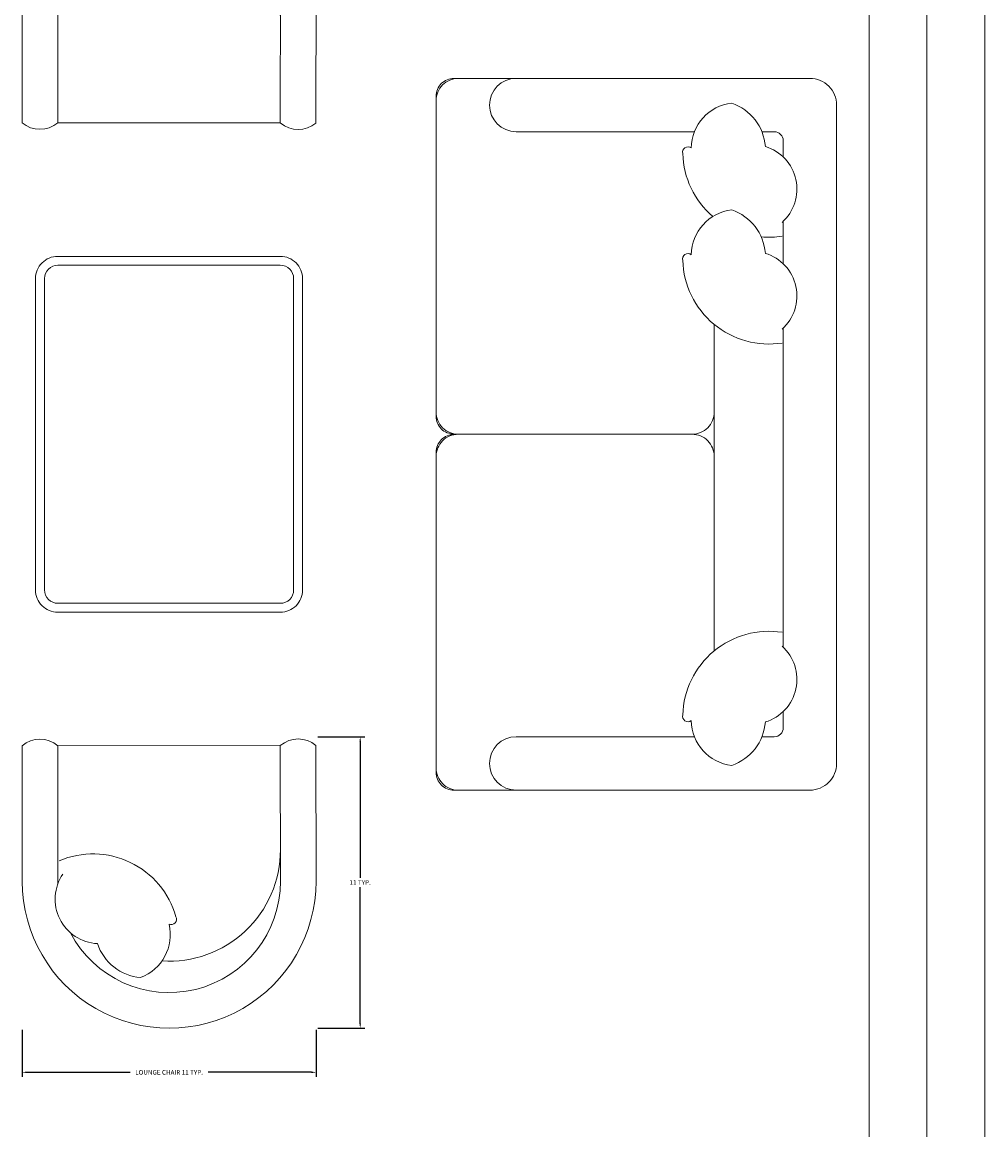
# Model space of a CAD drawing. Units: inches. Extents: x 1885 to 2748, y 783 to 2421.
# Tile 52 of 117: x 2410 to 2447, y 1764 to 1807. Entities that reach past the tile are written whole.
import ezdxf

# ---------------------------------------------------------------- set-up
doc = ezdxf.new("R2010")
doc.units = ezdxf.units.IN
for name, color, linetype, lineweight in [('A-ANNO-DIMS', 2, 'Continuous', 18), ('A-FURN', 8, 'Continuous', 13), ('A-GLAZ', 181, 'Continuous', 18)]:
    doc.layers.add(name, color=color, linetype=linetype, lineweight=lineweight)
doc.styles.get("Standard").update_dxf_attribs({"font": 'arial.ttf'})
doc.dimstyles.get("Standard").update_dxf_attribs({"dimtxt": 0.18, "dimasz": 0.18, "dimexe": 0.18, "dimexo": 0.0625, "dimgap": 0.09, "dimtad": 0, "dimtih": 1, "dimtoh": 1, "dimdec": 4, "dimzin": 0, "dimdsep": 46, "dimtxsty": 'Standard', "dimcen": 0.09, "dimadec": 0, "dimazin": 0, "dimtfac": 1, "dimtdec": 4, "dimtofl": 0, "dimtmove": 0, "dimatfit": 3, "dimfxl": 1, "dimtolj": 1, "dimtzin": 0, "dimarcsym": 0})

# ---------------------------------------------------------------- blocks, each defined once
blk = doc.blocks.new('A$C1352')
at = {"color": 0}
for points in [[(0.0027, 0.053), (0.0027, 0.553, -0.414214), (0.0527, 0.603), (0.7527, 0.603, -0.414214), (0.8027, 0.553), (0.8027, 0.053, -0.414214), (0.7527, 0.003), (0.0527, 0.003, -0.414214)], [(0.0227, 0.053), (0.0227, 0.553, -0.414214), (0.0527, 0.583), (0.7527, 0.583, -0.414214), (0.7827, 0.553), (0.7827, 0.053, -0.414214), (0.7527, 0.023), (0.0527, 0.023, -0.414214)]]:
    blk.add_lwpolyline(points, format="xyb", close=True, dxfattribs=at)
blk = doc.blocks.new('CHAIR-LOUNGE')
blk.add_line((1.388, 5.701), (1.383, 10.98))
at = {"ltscale": 0.03}
blk.add_lwpolyline([(1.383, 10.98, 0.369229), (-0.002, 10.979), (0.003, 5.7, 1), (11.423, 5.711), (11.418, 10.99, 0.369229), (10.034, 10.988)], format="xyb", close=True, dxfattribs=at)
blk.add_lwpolyline([(1.877, 3.707, 0.785087), (10.039, 5.71), (10.034, 10.988)], format="xyb")
for centre, radius, start, end in [((5.712, 6.928), 4.326, 266.342, 0.0539), ((2.748, 3.424), 3.35, 15.7143, 112.9857), ((3.014, 5.016), 1.734, 145.8599, 267.0078), ((5.713, 5.706), 4.326, 180.0539, 181.1464), ((5.792, 4.23), 0.207, 246.2577, 29.3762), ((3.979, 3.63), 1.778, 290.5305, 13.3597), ((4.772, 3.909), 1.951, 198.6466, 265.0001)]:
    blk.add_arc(centre, radius, start, end)
blk = doc.blocks.new('WIN-60')
for p, q in [((0.004, 59.998), (4.504, 59.998)), ((0.004, 59.998), (0.004, -0.002)), ((4.504, 59.998), (2.254, 59.998)), ((2.254, 59.998), (2.254, -0.002)), ((4.504, -0.002), (4.504, 59.998)), ((2.254, -0.002), (0.004, -0.002)), ((0.004, -0.002), (4.504, -0.002))]:
    blk.add_line(p, q)
blk = doc.blocks.new('*D33')
at = {"layer": 'A-ANNO-DIMS', "color": 0, "lineweight": -2, "transparency": 16777216}
for p, q in [((2409.848, 1767.42), (2409.848, 1765.589)), ((2421.276, 1767.42), (2421.276, 1765.589)), ((2410.028, 1765.769), (2414.046, 1765.769)), ((2421.096, 1765.769), (2417.078, 1765.769))]:
    blk.add_line(p, q, dxfattribs=at)
at = {"layer": 'A-ANNO-DIMS', "color": 0, "transparency": 16777216}
for points in [[(2410.028, 1765.799), (2410.028, 1765.739), (2409.848, 1765.769)], [(2421.096, 1765.799), (2421.096, 1765.739), (2421.276, 1765.769)]]:
    blk.add_solid(points, dxfattribs=at)
at = {"layer": 'Defpoints', "color": 0, "transparency": 16777216}
for p in [(2409.848, 1767.483), (2421.276, 1767.483), (2421.276, 1765.769)]:
    blk.add_point(p, dxfattribs=at)
at = {"layer": 'A-ANNO-DIMS', "color": 0, "transparency": 16777216, "insert": (2415.562, 1765.769), "char_height": 0.18, "attachment_point": 5}
blk.add_mtext('\\A1;LOUNGE CHAIR 11 TYP.', dxfattribs=at)
blk = doc.blocks.new('*D34')
at = {"layer": 'A-ANNO-DIMS', "color": 0, "lineweight": -2, "transparency": 16777216}
for p, q in [((2421.339, 1778.82), (2423.17, 1778.82)), ((2422.99, 1778.64), (2422.99, 1773.332)), ((2422.99, 1767.663), (2422.99, 1772.971)), ((2421.339, 1767.483), (2423.17, 1767.483))]:
    blk.add_line(p, q, dxfattribs=at)
at = {"layer": 'A-ANNO-DIMS', "color": 0, "transparency": 16777216}
for points in [[(2422.96, 1778.64), (2423.02, 1778.64), (2422.99, 1778.82)], [(2422.96, 1767.663), (2423.02, 1767.663), (2422.99, 1767.483)]]:
    blk.add_solid(points, dxfattribs=at)
at = {"layer": 'Defpoints', "color": 0, "transparency": 16777216}
for p in [(2421.276, 1778.82), (2422.99, 1778.82), (2421.276, 1767.483)]:
    blk.add_point(p, dxfattribs=at)
at = {"layer": 'A-ANNO-DIMS', "color": 0, "transparency": 16777216, "insert": (2422.99, 1773.151), "char_height": 0.18, "attachment_point": 5}
blk.add_mtext('\\A1;11 TYP.', dxfattribs=at)

msp = doc.modelspace()

# ---------------------------------------------------------------- linework, layer by layer
at = {"layer": 'A-FURN'}
for p, q in [((2435.981, 1802.352), (2429.054, 1802.352)), ((2438.608, 1802.352), (2439.09, 1802.352)), ((2439.436, 1802.006), (2439.436, 1801.369)), ((2439.436, 1797.215), (2439.436, 1798.871)), ((2439.436, 1797.851), (2439.436, 1797.215)), ((2439.436, 1782.301), (2439.436, 1794.717)), ((2439.436, 1779.166), (2439.436, 1779.803)), ((2429.054, 1778.82), (2435.981, 1778.82)), ((2438.608, 1778.82), (2439.09, 1778.82))]:
    msp.add_line(p, q, dxfattribs=at)
at = {"layer": 'A-FURN', "ltscale": 0.03}
msp.add_lwpolyline([(2426.632, 1790.577, 0.414214), (2425.94, 1789.885), (2425.94, 1777.436, 0.414214), (2426.632, 1776.744), (2440.474, 1776.744, 0.414214), (2441.512, 1777.782), (2441.512, 1803.39, 0.414214), (2440.474, 1804.428), (2426.632, 1804.428, 0.414214), (2425.94, 1803.736), (2425.94, 1791.287, 0.414214), (2426.632, 1790.594)], format="xyb", dxfattribs=at)
at = {"layer": 'A-FURN'}
for points in [[(2436.754, 1794.856), (2436.754, 1791.451, -0.414214), (2435.889, 1790.586), (2426.805, 1790.586, -0.414214), (2425.94, 1791.451), (2425.94, 1803.563, -0.414214), (2426.805, 1804.428)], [(2436.754, 1782.751), (2436.754, 1789.721, 0.414214), (2435.889, 1790.586), (2426.805, 1790.586, 0.414214), (2425.94, 1789.721), (2425.94, 1777.609, 0.414214), (2426.805, 1776.744)]]:
    msp.add_lwpolyline(points, format="xyb", dxfattribs=at)
msp.add_lwpolyline([(2436.754, 1794.856), (2436.754, 1782.162)], dxfattribs=at)
for centre, radius, start, end in [((2429.054, 1803.39), 1.038, 90, 180), ((2429.054, 1803.39), 1.038, 180, 270), ((2437.636, 1801.699), 1.778, 96.4279, 179.257), ((2436.798, 1801.622), 1.951, 4.5439, 70.8974), ((2439.09, 1802.006), 0.346, 0, 90), ((2439.09, 1802.006), 0.346, 0, 90), ((2435.731, 1801.559), 0.207, 52.155, 195.2735), ((2438.879, 1801.599), 3.35, 181.6116, 229.376), ((2438.234, 1800.12), 1.734, 311.7572, 72.9051), ((2437.636, 1797.545), 1.778, 96.4279, 179.257), ((2436.798, 1797.468), 1.951, 4.5439, 70.8974), ((2438.879, 1801.599), 3.35, 264.881, 278.883), ((2435.731, 1797.405), 0.207, 52.155, 195.2735), ((2438.234, 1795.966), 1.734, 311.7572, 72.9051), ((2438.879, 1797.445), 3.35, 181.6116, 278.883), ((2438.879, 1779.573), 3.35, 81.117, 178.3884), ((2438.234, 1781.052), 1.734, 287.0949, 48.2428), ((2435.731, 1779.613), 0.207, 164.7265, 307.845), ((2437.636, 1779.472), 1.778, 180.743, 263.5721), ((2436.798, 1779.55), 1.951, 289.1026, 355.4561), ((2439.09, 1779.166), 0.346, 270, 0), ((2429.054, 1777.782), 1.038, 90, 180), ((2429.054, 1777.782), 1.038, 180, 270)]:
    msp.add_arc(centre, radius, start, end, dxfattribs=at)

# ---------------------------------------------------------------- block references
at = {"layer": 'A-FURN', "extrusion": (0, 0, -1), "zscale": -1, "rotation": 180}
msp.add_blockref('CHAIR-LOUNGE', (-2409.85, 1813.682), dxfattribs=at)
at = {"layer": 'A-FURN', "ltscale": 0.03, "xscale": 17.30251319894821, "yscale": 17.30251319894821, "zscale": 17.30251319894821, "rotation": 270}
msp.add_blockref('A$C1352', (2410.316, 1797.553), dxfattribs=at)
at = {"layer": 'A-FURN'}
msp.add_blockref('CHAIR-LOUNGE', (2409.85, 1767.49), dxfattribs=at)
at = {"layer": 'A-GLAZ', "extrusion": (0, 0, -1), "zscale": -1, "rotation": 180}
msp.add_blockref('WIN-60', (-2442.77, 1809.268), dxfattribs=at)

# ---------------------------------------------------------------- dimensions: what is measured, and where the dimension line sits
at = {"layer": 'A-ANNO-DIMS'}
dim = msp.add_linear_dim(base=(2422.99, 1778.82), p1=(2421.276, 1767.483), p2=(2421.276, 1778.82), angle=90, text='<> TYP.', dimstyle='Standard', override={"dimdec": 0, "dimlfac": 1, "dimrnd": 0, "dimzin": 0, "dimdsep": 46, "dimlunit": 2}, dxfattribs=at)
dim.commit()
dim.dimension.update_dxf_attribs({"geometry": '*D34', "text_midpoint": (2422.99, 1773.151)})
dim = msp.add_linear_dim(base=(2421.276, 1765.769), p1=(2409.848, 1767.483), p2=(2421.276, 1767.483), text='LOUNGE CHAIR <> TYP.', dimstyle='Standard', override={"dimdec": 0, "dimlfac": 1, "dimrnd": 0, "dimzin": 0, "dimdsep": 46, "dimlunit": 2}, dxfattribs=at)
dim.commit()
dim.dimension.update_dxf_attribs({"geometry": '*D33', "text_midpoint": (2415.562, 1765.769)})

doc.saveas('drawing.dxf')
